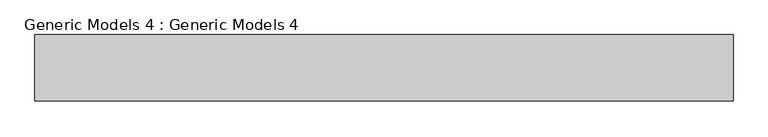
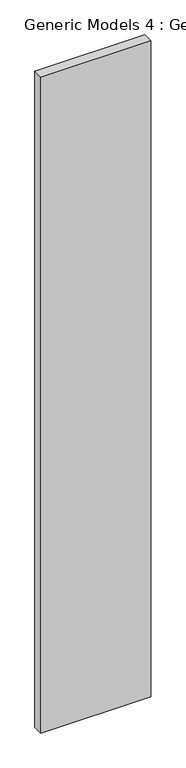
"""IFC4 building model written with IfcOpenShell, lengths in millimetres: proxy geometry, Generic Models 4 : Generic Models 4."""

from ifc_helpers import new_model, si_unit, frame, origin, place, context, project, spatial, polyline, outline, extrude, source, transform, mapped, element, save


def generic_models_4_generic_models_4_e8a7c7c6(model_context):
    return source(origin(), model_context, "Body", "SweptSolid", [
        extrude(outline(polyline([(8948.2271331, -12826.6643494), (8948.2271331, -12928.2643494), (7881.4271331, -12928.2643494), (7881.4271331, -12826.6643494), (8948.2271331, -12826.6643494)])), frame((0.0, 0.0, 4419.6), z_axis=(0.0, 0.0, 1.0), x_axis=(1.0, 0.0, 0.0)), (0.0, 0.0, 1.0), 6731.0),
    ])


if __name__ == "__main__":
    model = new_model("IFC4")
    model_context = context("Model", 3, world=origin())
    ifc_project = project(units=[si_unit("LENGTHUNIT", "METRE", prefix="MILLI")], contexts=[model_context])
    site = spatial("IfcSite", under=ifc_project)
    building = spatial("IfcBuilding", under=site)
    placement = place(None, origin())
    generic_models_4_generic_models_4_shape = generic_models_4_generic_models_4_e8a7c7c6(model_context)
    element("IfcBuildingElementProxy", 1, Name="Generic Models 4 : Generic Models 4", ObjectType="Generic Models 4 : Generic Models 4", at=placement, inside=building, context=model_context, shape_type="MappedRepresentation", body=[
        mapped(generic_models_4_generic_models_4_shape, transform((0.0, 0.0, 0.0), x_axis=(1.0, 0.0, 0.0), y_axis=(0.0, 1.0, 0.0), z_axis=(0.0, 0.0, 1.0))),
    ])
    save(model, "model.ifc")
